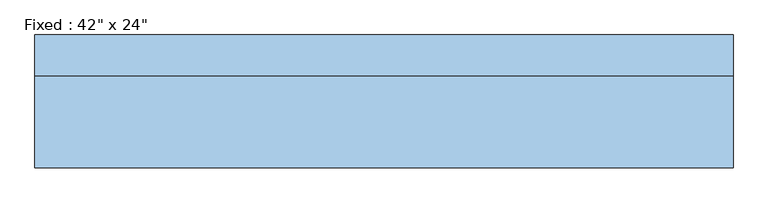
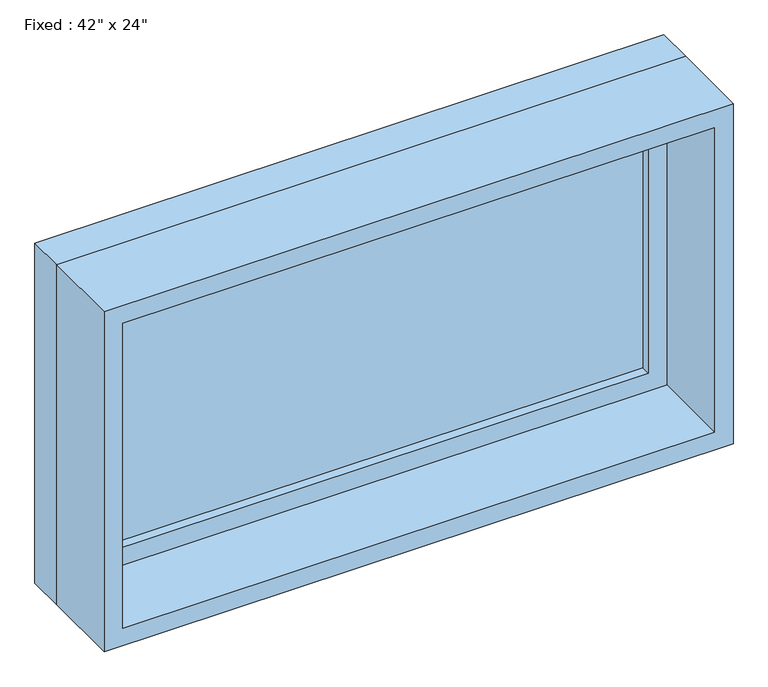
"""IFC4 building model written with IfcOpenShell, lengths in millimetres: window geometry."""

from ifc_helpers import new_model, si_unit, frame, origin, place, context, project, spatial, polyline, outline, extrude, source, transform, mapped, element, save


def window_e8893895(model_context):
    return source(origin(), model_context, "Body", "SweptSolid", [
        extrude(outline(polyline([(431.8, 53.975), (-508.0, 53.975), (-508.0, 66.675), (431.8, 66.675), (431.8, 53.975)])), frame((0.0, 0.0, 2197.1), z_axis=(0.0, 0.0, 1.0), x_axis=(1.0, 0.0, 0.0)), (0.0, 0.0, 1.0), 482.6),
        extrude(outline(polyline([(2724.15, -552.45), (2152.65, -552.45), (2152.65, 476.25), (2724.15, 476.25), (2724.15, -552.45)]), holes=[polyline([(2679.7, -508.0), (2679.7, 431.8), (2197.1, 431.8), (2197.1, -508.0), (2679.7, -508.0)])]), frame((0.0, 38.1, 0.0), z_axis=(0.0, 1.0, 0.0), x_axis=(0.0, 0.0, 1.0)), (0.0, 0.0, 1.0), 44.45),
        extrude(outline(polyline([(2743.2, -571.5), (2133.6, -571.5), (2133.6, 495.3), (2743.2, 495.3), (2743.2, -571.5)]), holes=[polyline([(2711.45, -539.75), (2711.45, 463.55), (2165.35, 463.55), (2165.35, -539.75), (2711.45, -539.75)])]), frame((0.0, -101.6, 0.0), z_axis=(0.0, 1.0, 0.0), x_axis=(0.0, 0.0, 1.0)), (0.0, 0.0, 1.0), 139.7),
        extrude(outline(polyline([(2743.2, 495.3), (2743.2, -571.5), (2133.6, -571.5), (2133.6, 495.3), (2743.2, 495.3)]), holes=[polyline([(2724.15, 476.25), (2152.65, 476.25), (2152.65, -552.45), (2724.15, -552.45), (2724.15, 476.25)])]), frame((0.0, 38.1, 0.0), z_axis=(0.0, 1.0, 0.0), x_axis=(0.0, 0.0, 1.0)), (0.0, 0.0, 1.0), 63.5),
    ])


if __name__ == "__main__":
    model = new_model("IFC4")
    model_context = context("Model", 3, world=origin())
    ifc_project = project(units=[si_unit("LENGTHUNIT", "METRE", prefix="MILLI")], contexts=[model_context])
    site = spatial("IfcSite", under=ifc_project)
    building = spatial("IfcBuilding", under=site)
    placement = place(None, origin())
    window_shape = window_e8893895(model_context)
    element("IfcWindow", 1, ObjectType="Fixed : 42\" x 24\"", at=placement, inside=building, context=model_context, shape_type="MappedRepresentation", body=[
        mapped(window_shape, transform((0.0, 0.0, 0.0), x_axis=(1.0, 0.0, 0.0), y_axis=(0.0, 1.0, 0.0), z_axis=(0.0, 0.0, 1.0))),
    ])
    save(model, "model.ifc")

# Revit data of these elements
# Type "Fixed : 42\" x 24\""
#   Type Mark = "18"
#   Construction Type Id = "GSP4R"
#   Assembly Code = "B2020100"
#   Analytic Construction = "1/8 in Pilkington single glazing"
#   Visual Light Transmittance = 0.9
#   Solar Heat Gain Coefficient = 0.78
#   Heat Transfer Coefficient (U) = 0.6496 BTU/(h·ft²·°F)
#   Height = 2' - 0"
#   Default Sill Height = 7' - 0"
#   Width = 3' - 6"
#   Window Inset = 0' - 0 3/4"
#   Define Thermal Properties by = 1
#   Glass Pane Material = Glass
#   Sash Material = Sash
#   Wall Closure = (empty or 0)
# Element 1 (IfcWindow, "Fixed : 42\" x 24\"")
#   Materials on its faces: "Sash", "Glass"
# Materials
#   "Glass": class "Glass", colour RGB 0 128 192, transparency 0.75, Description = "Soda Lime Glass", Cost = 0
#   "Sash": class "Wood", colour RGB 224 178 126, transparency 0, Cost = 0
